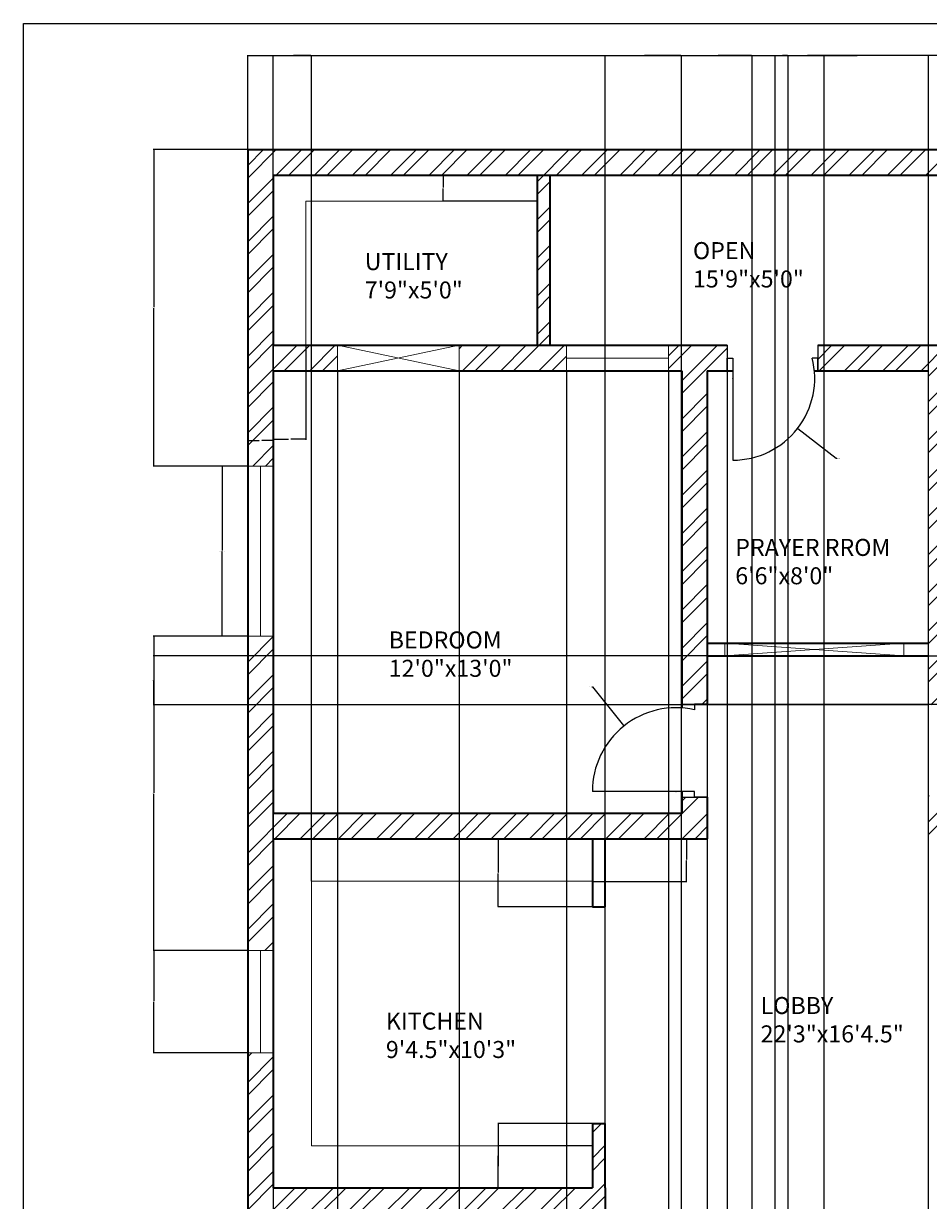
# Model space of a CAD drawing. Units: inches. Extents: x 1595 to 2135, y 460 to 2061.
# Tile 4 of 5: x 1595 to 1914, y 1646 to 2061. Entities that reach past the tile are written whole.
import ezdxf

# ---------------------------------------------------------------- set-up
doc = ezdxf.new("R2010")
doc.units = ezdxf.units.IN
for name, color, linetype, lineweight in [('A-ANNO-DIMS', 2, 'Continuous', 18), ('A-ANNO-TTLB', 7, 'Continuous', 25), ('A-AREA-IDEN', 7, 'Continuous', 18), ('A-DOOR', 3, 'Continuous', 25), ('A-FLOR-FIXT', 9, 'Continuous', 18), ('A-GLAZ', 4, 'Continuous', 18), ('A-WALL', 7, 'Continuous', 35)]:
    doc.layers.add(name, color=color, linetype=linetype, lineweight=lineweight)
doc.layers.add('A-WALL-PATT', color=143, linetype='Continuous', lineweight=13, true_color=0x7aafdf)
doc.styles.get("Standard").update_dxf_attribs({"font": 'arial.ttf'})
doc.dimstyles.get("Standard").update_dxf_attribs({"dimtxt": 0.18, "dimasz": 0.18, "dimexe": 0.18, "dimexo": 0.0625, "dimgap": 0.09, "dimtad": 0, "dimtih": 1, "dimtoh": 1, "dimdec": 4, "dimzin": 0, "dimdsep": 46, "dimtxsty": 'Standard', "dimcen": 0.09, "dimadec": 0, "dimazin": 0, "dimtfac": 1, "dimtdec": 4, "dimtofl": 0, "dimtmove": 0, "dimatfit": 3, "dimfxl": 1, "dimtolj": 1, "dimtzin": 0, "dimarcsym": 0})

# ---------------------------------------------------------------- blocks, each defined once
blk = doc.blocks.new('WIN-60IN')
for p, q in [((4.5, 60), (0, 60)), ((0, 60), (9, 60)), ((4.5, 0), (4.5, 60)), ((0, 0), (9, 0)), ((9, 0), (4.5, 0))]:
    blk.add_line(p, q)
blk = doc.blocks.new('*D2')
at = {"layer": 'A-ANNO-DIMS', "color": 0, "lineweight": -2, "transparency": 16777216}
for p, q in [((1674.25, 1905.07), (1665.13, 1905.07)), ((1665.31, 1904.89), (1665.31, 1875.26)), ((1665.31, 1845.25), (1665.31, 1874.89)), ((1674.25, 1845.07), (1665.13, 1845.07))]:
    blk.add_line(p, q, dxfattribs=at)
at = {"layer": 'A-ANNO-DIMS', "color": 0, "transparency": 16777216}
for points in [[(1665.28, 1904.89), (1665.34, 1904.89), (1665.31, 1905.07)], [(1665.28, 1845.25), (1665.34, 1845.25), (1665.31, 1845.07)]]:
    blk.add_solid(points, dxfattribs=at)
at = {"layer": 'Defpoints', "color": 0, "transparency": 16777216}
for p in [(1674.31, 1905.07), (1665.31, 1845.07), (1674.31, 1845.07)]:
    blk.add_point(p, dxfattribs=at)
at = {"layer": 'A-ANNO-DIMS', "color": 0, "transparency": 16777216, "insert": (1665.31, 1875.07), "char_height": 0.18, "attachment_point": 5}
blk.add_mtext('\\A1;WINDOW 60 TYP.', dxfattribs=at)
blk = doc.blocks.new('*D3')
at = {"layer": 'A-ANNO-DIMS', "color": 0, "lineweight": -2, "transparency": 16777216}
for p, q in [((1674.31, 1905.14), (1674.31, 1914.25)), ((1674.49, 1914.07), (1678.35, 1914.07)), ((1683.13, 1914.07), (1679.27, 1914.07)), ((1683.31, 1905.14), (1683.31, 1914.25))]:
    blk.add_line(p, q, dxfattribs=at)
at = {"layer": 'A-ANNO-DIMS', "color": 0, "transparency": 16777216}
for points in [[(1674.49, 1914.1), (1674.49, 1914.04), (1674.31, 1914.07)], [(1683.13, 1914.1), (1683.13, 1914.04), (1683.31, 1914.07)]]:
    blk.add_solid(points, dxfattribs=at)
at = {"layer": 'Defpoints', "color": 0, "transparency": 16777216}
for p in [(1674.31, 1914.07), (1674.31, 1905.07), (1683.31, 1905.07)]:
    blk.add_point(p, dxfattribs=at)
at = {"layer": 'A-ANNO-DIMS', "color": 0, "transparency": 16777216, "insert": (1678.81, 1914.07), "char_height": 0.18, "attachment_point": 5}
blk.add_mtext('\\A1;9 TYP.', dxfattribs=at)
blk = doc.blocks.new('*D4')
at = {"layer": 'A-ANNO-DIMS', "color": 0, "lineweight": -2, "transparency": 16777216}
for p, q in [((1795.75, 1773.64), (1762.48, 1773.64)), ((1762.66, 1773.46), (1762.66, 1761.82)), ((1762.66, 1749.81), (1762.66, 1761.46)), ((1795.75, 1749.63), (1762.48, 1749.63))]:
    blk.add_line(p, q, dxfattribs=at)
at = {"layer": 'A-ANNO-DIMS', "color": 0, "transparency": 16777216}
for points in [[(1762.63, 1773.46), (1762.69, 1773.46), (1762.66, 1773.64)], [(1762.63, 1749.81), (1762.69, 1749.81), (1762.66, 1749.63)]]:
    blk.add_solid(points, dxfattribs=at)
at = {"layer": 'Defpoints', "color": 0, "transparency": 16777216}
for p in [(1762.66, 1773.64), (1795.81, 1773.64), (1795.81, 1749.63)]:
    blk.add_point(p, dxfattribs=at)
at = {"layer": 'A-ANNO-DIMS', "color": 0, "transparency": 16777216, "insert": (1762.66, 1761.64), "char_height": 0.18, "attachment_point": 5}
blk.add_mtext('\\A1;24.01', dxfattribs=at)
blk = doc.blocks.new('*D5')
at = {"layer": 'A-ANNO-DIMS', "color": 0, "lineweight": -2, "transparency": 16777216}
for p, q in [((1795.75, 1673.31), (1762.48, 1673.31)), ((1762.66, 1673.13), (1762.66, 1662.16)), ((1762.66, 1650.82), (1762.66, 1661.79)), ((1795.75, 1650.64), (1762.48, 1650.64))]:
    blk.add_line(p, q, dxfattribs=at)
at = {"layer": 'A-ANNO-DIMS', "color": 0, "transparency": 16777216}
for points in [[(1762.63, 1673.13), (1762.69, 1673.13), (1762.66, 1673.31)], [(1762.63, 1650.82), (1762.69, 1650.82), (1762.66, 1650.64)]]:
    blk.add_solid(points, dxfattribs=at)
at = {"layer": 'Defpoints', "color": 0, "transparency": 16777216}
for p in [(1762.66, 1673.31), (1795.81, 1673.31), (1795.81, 1650.64)]:
    blk.add_point(p, dxfattribs=at)
at = {"layer": 'A-ANNO-DIMS', "color": 0, "transparency": 16777216, "insert": (1762.66, 1661.97), "char_height": 0.18, "attachment_point": 5}
blk.add_mtext('\\A1;22.663', dxfattribs=at)
blk = doc.blocks.new('*D11')
at = {"layer": 'A-ANNO-DIMS', "color": 0, "lineweight": -2, "transparency": 16777216}
for p, q in [((1674.25, 2016.64), (1640.98, 2016.64)), ((1641.16, 2016.46), (1641.16, 1961.04)), ((1641.16, 1905.25), (1641.16, 1960.68)), ((1674.25, 1905.07), (1640.98, 1905.07))]:
    blk.add_line(p, q, dxfattribs=at)
at = {"layer": 'A-ANNO-DIMS', "color": 0, "transparency": 16777216}
for points in [[(1641.13, 2016.46), (1641.19, 2016.46), (1641.16, 2016.64)], [(1641.13, 1905.25), (1641.19, 1905.25), (1641.16, 1905.07)]]:
    blk.add_solid(points, dxfattribs=at)
at = {"layer": 'Defpoints', "color": 0, "transparency": 16777216}
for p in [(1674.31, 2016.64), (1641.16, 1905.07), (1674.31, 1905.07)]:
    blk.add_point(p, dxfattribs=at)
at = {"layer": 'A-ANNO-DIMS', "color": 0, "transparency": 16777216, "insert": (1641.16, 1960.86), "char_height": 0.18, "attachment_point": 5}
blk.add_mtext('\\A1;111.57', dxfattribs=at)
blk = doc.blocks.new('*D12')
at = {"layer": 'A-ANNO-DIMS', "color": 0, "lineweight": -2, "transparency": 16777216}
for p, q in [((1674.25, 1734.21), (1640.98, 1734.21)), ((1641.16, 1734.03), (1641.16, 1716.39)), ((1641.16, 1698.39), (1641.16, 1716.03)), ((1674.25, 1698.21), (1640.98, 1698.21))]:
    blk.add_line(p, q, dxfattribs=at)
at = {"layer": 'A-ANNO-DIMS', "color": 0, "transparency": 16777216}
for points in [[(1641.13, 1734.03), (1641.19, 1734.03), (1641.16, 1734.21)], [(1641.13, 1698.39), (1641.19, 1698.39), (1641.16, 1698.21)]]:
    blk.add_solid(points, dxfattribs=at)
at = {"layer": 'Defpoints', "color": 0, "transparency": 16777216}
for p in [(1674.31, 1734.21), (1641.16, 1698.21), (1674.31, 1698.21)]:
    blk.add_point(p, dxfattribs=at)
at = {"layer": 'A-ANNO-DIMS', "color": 0, "transparency": 16777216, "insert": (1641.16, 1716.21), "char_height": 0.18, "attachment_point": 5}
blk.add_mtext('\\A1;36', dxfattribs=at)
blk = doc.blocks.new('*D13')
at = {"layer": 'A-ANNO-DIMS', "color": 0, "lineweight": -2, "transparency": 16777216}
for p, q in [((1674.25, 1845.07), (1640.98, 1845.07)), ((1641.16, 1844.89), (1641.16, 1789.82)), ((1641.16, 1734.39), (1641.16, 1789.46)), ((1674.25, 1734.21), (1640.98, 1734.21))]:
    blk.add_line(p, q, dxfattribs=at)
at = {"layer": 'A-ANNO-DIMS', "color": 0, "transparency": 16777216}
for points in [[(1641.13, 1844.89), (1641.19, 1844.89), (1641.16, 1845.07)], [(1641.13, 1734.39), (1641.19, 1734.39), (1641.16, 1734.21)]]:
    blk.add_solid(points, dxfattribs=at)
at = {"layer": 'Defpoints', "color": 0, "transparency": 16777216}
for p in [(1674.31, 1845.07), (1641.16, 1734.21), (1674.31, 1734.21)]:
    blk.add_point(p, dxfattribs=at)
at = {"layer": 'A-ANNO-DIMS', "color": 0, "transparency": 16777216, "insert": (1641.16, 1789.64), "char_height": 0.18, "attachment_point": 5}
blk.add_mtext('\\A1;110.86', dxfattribs=at)
blk = doc.blocks.new('*D23')
at = {"layer": 'A-ANNO-DIMS', "color": 0, "lineweight": -2, "transparency": 16777216}
for p, q in [((1683.31, 1938.58), (1683.31, 1365.31)), ((1705.98, 1938.58), (1705.98, 1365.31)), ((1683.49, 1365.49), (1694.18, 1365.49)), ((1705.8, 1365.49), (1695.11, 1365.49))]:
    blk.add_line(p, q, dxfattribs=at)
at = {"layer": 'A-ANNO-DIMS', "color": 0, "transparency": 16777216}
for points in [[(1683.49, 1365.52), (1683.49, 1365.46), (1683.31, 1365.49)], [(1705.8, 1365.52), (1705.8, 1365.46), (1705.98, 1365.49)]]:
    blk.add_solid(points, dxfattribs=at)
at = {"layer": 'Defpoints', "color": 0, "transparency": 16777216}
for p in [(1683.31, 1938.64), (1705.98, 1938.64), (1705.98, 1365.49)]:
    blk.add_point(p, dxfattribs=at)
at = {"layer": 'A-ANNO-DIMS', "color": 0, "transparency": 16777216, "insert": (1694.64, 1365.49), "char_height": 0.18, "attachment_point": 5}
blk.add_mtext('\\A1;22.663', dxfattribs=at)
blk = doc.blocks.new('*D24')
at = {"layer": 'A-ANNO-DIMS', "color": 0, "lineweight": -2, "transparency": 16777216}
for p, q in [((1705.98, 1938.58), (1705.98, 1365.31)), ((1748.87, 1938.58), (1748.87, 1365.31)), ((1706.16, 1365.49), (1726.96, 1365.49)), ((1748.69, 1365.49), (1727.89, 1365.49))]:
    blk.add_line(p, q, dxfattribs=at)
at = {"layer": 'A-ANNO-DIMS', "color": 0, "transparency": 16777216}
for points in [[(1706.16, 1365.52), (1706.16, 1365.46), (1705.98, 1365.49)], [(1748.69, 1365.52), (1748.69, 1365.46), (1748.87, 1365.49)]]:
    blk.add_solid(points, dxfattribs=at)
at = {"layer": 'Defpoints', "color": 0, "transparency": 16777216}
for p in [(1705.98, 1938.64), (1748.87, 1938.64), (1748.87, 1365.49)]:
    blk.add_point(p, dxfattribs=at)
at = {"layer": 'A-ANNO-DIMS', "color": 0, "transparency": 16777216, "insert": (1727.42, 1365.49), "char_height": 0.18, "attachment_point": 5}
blk.add_mtext('\\A1;42.894', dxfattribs=at)
blk = doc.blocks.new('*D25')
at = {"layer": 'A-ANNO-DIMS', "color": 0, "lineweight": -2, "transparency": 16777216}
for p, q in [((1748.87, 1938.58), (1748.87, 1365.31)), ((1786.65, 1938.58), (1786.65, 1365.31)), ((1749.05, 1365.49), (1767.37, 1365.49)), ((1786.47, 1365.49), (1768.16, 1365.49))]:
    blk.add_line(p, q, dxfattribs=at)
at = {"layer": 'A-ANNO-DIMS', "color": 0, "transparency": 16777216}
for points in [[(1749.05, 1365.52), (1749.05, 1365.46), (1748.87, 1365.49)], [(1786.47, 1365.52), (1786.47, 1365.46), (1786.65, 1365.49)]]:
    blk.add_solid(points, dxfattribs=at)
at = {"layer": 'Defpoints', "color": 0, "transparency": 16777216}
for p in [(1748.87, 1938.64), (1786.65, 1938.64), (1786.65, 1365.49)]:
    blk.add_point(p, dxfattribs=at)
at = {"layer": 'A-ANNO-DIMS', "color": 0, "transparency": 16777216, "insert": (1767.76, 1365.49), "char_height": 0.18, "attachment_point": 5}
blk.add_mtext('\\A1;37.78', dxfattribs=at)
blk = doc.blocks.new('*D26')
at = {"layer": 'A-ANNO-DIMS', "color": 0, "lineweight": -2, "transparency": 16777216}
for p, q in [((1786.65, 1938.58), (1786.65, 1365.31)), ((1822.65, 1938.58), (1822.65, 1365.31)), ((1786.83, 1365.49), (1804.43, 1365.49)), ((1822.47, 1365.49), (1804.87, 1365.49))]:
    blk.add_line(p, q, dxfattribs=at)
at = {"layer": 'A-ANNO-DIMS', "color": 0, "transparency": 16777216}
for points in [[(1786.83, 1365.52), (1786.83, 1365.46), (1786.65, 1365.49)], [(1822.47, 1365.52), (1822.47, 1365.46), (1822.65, 1365.49)]]:
    blk.add_solid(points, dxfattribs=at)
at = {"layer": 'Defpoints', "color": 0, "transparency": 16777216}
for p in [(1786.65, 1938.64), (1822.65, 1938.64), (1822.65, 1365.49)]:
    blk.add_point(p, dxfattribs=at)
at = {"layer": 'A-ANNO-DIMS', "color": 0, "transparency": 16777216, "insert": (1804.65, 1365.49), "char_height": 0.18, "attachment_point": 5}
blk.add_mtext('\\A1;36', dxfattribs=at)
blk = doc.blocks.new('*D30')
at = {"layer": 'A-ANNO-DIMS', "color": 0, "lineweight": -2, "transparency": 16777216}
for p, q in [((1836.31, 1938.58), (1836.31, 1365.31)), ((1843.37, 1938.58), (1843.37, 1365.31)), ((1836.49, 1365.49), (1839.45, 1365.49)), ((1843.19, 1365.49), (1840.23, 1365.49))]:
    blk.add_line(p, q, dxfattribs=at)
at = {"layer": 'A-ANNO-DIMS', "color": 0, "transparency": 16777216}
for points in [[(1836.49, 1365.52), (1836.49, 1365.46), (1836.31, 1365.49)], [(1843.19, 1365.52), (1843.19, 1365.46), (1843.37, 1365.49)]]:
    blk.add_solid(points, dxfattribs=at)
at = {"layer": 'Defpoints', "color": 0, "transparency": 16777216}
for p in [(1836.31, 1938.64), (1843.37, 1938.64), (1843.37, 1365.49)]:
    blk.add_point(p, dxfattribs=at)
at = {"layer": 'A-ANNO-DIMS', "color": 0, "transparency": 16777216, "insert": (1839.84, 1365.49), "char_height": 0.18, "attachment_point": 5}
blk.add_mtext('\\A1;7.054', dxfattribs=at)
blk = doc.blocks.new('*D31')
at = {"layer": 'A-ANNO-DIMS', "color": 0, "lineweight": -2, "transparency": 16777216}
for p, q in [((1836.38, 1838.14), (2109.64, 1838.14)), ((2109.46, 1837.96), (2109.46, 1829.81)), ((2109.46, 1821.29), (2109.46, 1829.44)), ((1836.38, 1821.11), (2109.64, 1821.11))]:
    blk.add_line(p, q, dxfattribs=at)
at = {"layer": 'A-ANNO-DIMS', "color": 0, "transparency": 16777216}
for points in [[(2109.43, 1837.96), (2109.49, 1837.96), (2109.46, 1838.14)], [(2109.43, 1821.29), (2109.49, 1821.29), (2109.46, 1821.11)]]:
    blk.add_solid(points, dxfattribs=at)
at = {"layer": 'Defpoints', "color": 0, "transparency": 16777216}
for p in [(1836.31, 1838.14), (1836.31, 1821.11), (2109.46, 1821.11)]:
    blk.add_point(p, dxfattribs=at)
at = {"layer": 'A-ANNO-DIMS', "color": 0, "transparency": 16777216, "insert": (2109.46, 1829.63), "char_height": 0.18, "attachment_point": 5}
blk.add_mtext('\\A1;17.034', dxfattribs=at)
blk = doc.blocks.new('*D32')
at = {"layer": 'A-ANNO-DIMS', "color": 0, "lineweight": -2, "transparency": 16777216}
for p, q in [((1914.25, 1838.14), (1640.98, 1838.14)), ((1641.16, 1837.96), (1641.16, 1829.7)), ((1641.16, 1821.07), (1641.16, 1829.33)), ((1914.25, 1820.89), (1640.98, 1820.89))]:
    blk.add_line(p, q, dxfattribs=at)
at = {"layer": 'A-ANNO-DIMS', "color": 0, "transparency": 16777216}
for points in [[(1641.13, 1837.96), (1641.19, 1837.96), (1641.16, 1838.14)], [(1641.13, 1821.07), (1641.19, 1821.07), (1641.16, 1820.89)]]:
    blk.add_solid(points, dxfattribs=at)
at = {"layer": 'Defpoints', "color": 0, "transparency": 16777216}
for p in [(1914.31, 1838.14), (1641.16, 1820.89), (1914.31, 1820.89)]:
    blk.add_point(p, dxfattribs=at)
at = {"layer": 'A-ANNO-DIMS', "color": 0, "transparency": 16777216, "insert": (1641.16, 1829.52), "char_height": 0.18, "attachment_point": 5}
blk.add_mtext('\\A1;17.253', dxfattribs=at)
blk = doc.blocks.new('*D35')
at = {"layer": 'A-ANNO-DIMS', "color": 0, "lineweight": -2, "transparency": 16777216}
for p, q in [((1864.81, 1540.04), (1864.81, 2049.97)), ((1864.99, 2049.79), (1889.23, 2049.79)), ((1914.13, 2049.79), (1889.89, 2049.79)), ((1914.31, 1540.04), (1914.31, 2049.97))]:
    blk.add_line(p, q, dxfattribs=at)
at = {"layer": 'A-ANNO-DIMS', "color": 0, "transparency": 16777216}
for points in [[(1864.99, 2049.82), (1864.99, 2049.76), (1864.81, 2049.79)], [(1914.13, 2049.82), (1914.13, 2049.76), (1914.31, 2049.79)]]:
    blk.add_solid(points, dxfattribs=at)
at = {"layer": 'Defpoints', "color": 0, "transparency": 16777216}
for p in [(1914.31, 2049.79), (1864.81, 1539.98), (1914.31, 1539.98)]:
    blk.add_point(p, dxfattribs=at)
at = {"layer": 'A-ANNO-DIMS', "color": 0, "transparency": 16777216, "insert": (1889.56, 2049.79), "char_height": 0.18, "attachment_point": 5}
blk.add_mtext('\\A1;49.5', dxfattribs=at)
blk = doc.blocks.new('*D36')
at = {"layer": 'A-ANNO-DIMS', "color": 0, "lineweight": -2, "transparency": 16777216}
for p, q in [((1860.31, 1568.2), (1860.31, 2049.97)), ((1860.49, 2049.79), (1862.3, 2049.79)), ((1864.63, 2049.79), (1862.82, 2049.79)), ((1864.81, 1577.2), (1864.81, 2049.97))]:
    blk.add_line(p, q, dxfattribs=at)
at = {"layer": 'A-ANNO-DIMS', "color": 0, "transparency": 16777216}
for points in [[(1860.49, 2049.82), (1860.49, 2049.76), (1860.31, 2049.79)], [(1864.63, 2049.82), (1864.63, 2049.76), (1864.81, 2049.79)]]:
    blk.add_solid(points, dxfattribs=at)
at = {"layer": 'Defpoints', "color": 0, "transparency": 16777216}
for p in [(1864.81, 2049.79), (1864.81, 1577.14), (1860.31, 1568.14)]:
    blk.add_point(p, dxfattribs=at)
at = {"layer": 'A-ANNO-DIMS', "color": 0, "transparency": 16777216, "insert": (1862.56, 2049.79), "char_height": 0.18, "attachment_point": 5}
blk.add_mtext('\\A1;4.5', dxfattribs=at)
blk = doc.blocks.new('*D37')
at = {"layer": 'A-ANNO-DIMS', "color": 0, "lineweight": -2, "transparency": 16777216}
for p, q in [((1800.31, 1577.2), (1800.31, 2049.97)), ((1800.49, 2049.79), (1813.31, 2049.79)), ((1827.06, 2049.79), (1814.24, 2049.79)), ((1827.24, 1577.2), (1827.24, 2049.97))]:
    blk.add_line(p, q, dxfattribs=at)
at = {"layer": 'A-ANNO-DIMS', "color": 0, "transparency": 16777216}
for points in [[(1800.49, 2049.82), (1800.49, 2049.76), (1800.31, 2049.79)], [(1827.06, 2049.82), (1827.06, 2049.76), (1827.24, 2049.79)]]:
    blk.add_solid(points, dxfattribs=at)
at = {"layer": 'Defpoints', "color": 0, "transparency": 16777216}
for p in [(1827.24, 2049.79), (1800.31, 1577.14), (1827.24, 1577.14)]:
    blk.add_point(p, dxfattribs=at)
at = {"layer": 'A-ANNO-DIMS', "color": 0, "transparency": 16777216, "insert": (1813.78, 2049.79), "char_height": 0.18, "attachment_point": 5}
blk.add_mtext('\\A1;26.927', dxfattribs=at)
blk = doc.blocks.new('*D38')
at = {"layer": 'A-ANNO-DIMS', "color": 0, "lineweight": -2, "transparency": 16777216}
for p, q in [((1827.24, 1577.2), (1827.24, 2049.97)), ((1827.42, 2049.79), (1839.23, 2049.79)), ((1851.96, 2049.79), (1840.16, 2049.79)), ((1852.14, 1577.2), (1852.14, 2049.97))]:
    blk.add_line(p, q, dxfattribs=at)
at = {"layer": 'A-ANNO-DIMS', "color": 0, "transparency": 16777216}
for points in [[(1827.42, 2049.82), (1827.42, 2049.76), (1827.24, 2049.79)], [(1851.96, 2049.82), (1851.96, 2049.76), (1852.14, 2049.79)]]:
    blk.add_solid(points, dxfattribs=at)
at = {"layer": 'Defpoints', "color": 0, "transparency": 16777216}
for p in [(1852.14, 2049.79), (1827.24, 1577.14), (1852.14, 1577.14)]:
    blk.add_point(p, dxfattribs=at)
at = {"layer": 'A-ANNO-DIMS', "color": 0, "transparency": 16777216, "insert": (1839.69, 2049.79), "char_height": 0.18, "attachment_point": 5}
blk.add_mtext('\\A1;24.904', dxfattribs=at)
blk = doc.blocks.new('*D44')
at = {"layer": 'A-ANNO-DIMS', "color": 0, "lineweight": -2, "transparency": 16777216}
for p, q in [((1864.81, 1549.04), (1864.81, 2049.97)), ((1864.99, 2049.79), (1870.74, 2049.79)), ((1877.4, 2049.79), (1871.65, 2049.79)), ((1877.58, 1549.04), (1877.58, 2049.97))]:
    blk.add_line(p, q, dxfattribs=at)
at = {"layer": 'A-ANNO-DIMS', "color": 0, "transparency": 16777216}
for points in [[(1864.99, 2049.82), (1864.99, 2049.76), (1864.81, 2049.79)], [(1877.4, 2049.82), (1877.4, 2049.76), (1877.58, 2049.79)]]:
    blk.add_solid(points, dxfattribs=at)
at = {"layer": 'Defpoints', "color": 0, "transparency": 16777216}
for p in [(1877.58, 2049.79), (1864.81, 1548.98), (1877.58, 1548.98)]:
    blk.add_point(p, dxfattribs=at)
at = {"layer": 'A-ANNO-DIMS', "color": 0, "transparency": 16777216, "insert": (1871.2, 2049.79), "char_height": 0.18, "attachment_point": 5}
blk.add_mtext('\\A1;12.769', dxfattribs=at)
blk = doc.blocks.new('*D45')
at = {"layer": 'A-ANNO-DIMS', "color": 0, "lineweight": -2, "transparency": 16777216}
for p, q in [((1674.31, 2016.7), (1674.31, 2049.97)), ((1674.49, 2049.79), (1875.02, 2049.79)), ((2076.13, 2049.79), (1875.6, 2049.79)), ((2076.31, 2016.7), (2076.31, 2049.97))]:
    blk.add_line(p, q, dxfattribs=at)
at = {"layer": 'A-ANNO-DIMS', "color": 0, "transparency": 16777216}
for points in [[(1674.49, 2049.82), (1674.49, 2049.76), (1674.31, 2049.79)], [(2076.13, 2049.82), (2076.13, 2049.76), (2076.31, 2049.79)]]:
    blk.add_solid(points, dxfattribs=at)
at = {"layer": 'Defpoints', "color": 0, "transparency": 16777216}
for p in [(2076.31, 2049.79), (1674.31, 2016.64), (2076.31, 2016.64)]:
    blk.add_point(p, dxfattribs=at)
at = {"layer": 'A-ANNO-DIMS', "color": 0, "transparency": 16777216, "insert": (1875.31, 2049.79), "char_height": 0.18, "attachment_point": 5}
blk.add_mtext('\\A1;402', dxfattribs=at)
blk = doc.blocks.new('*D49')
at = {"layer": 'A-ANNO-DIMS', "color": 0, "lineweight": -2, "transparency": 16777216}
for p, q in [((1683.31, 1947.58), (1683.31, 1914.31)), ((1694.85, 1947.58), (1694.85, 1914.31)), ((1683.49, 1914.49), (1688.7, 1914.49)), ((1694.67, 1914.49), (1689.47, 1914.49))]:
    blk.add_line(p, q, dxfattribs=at)
at = {"layer": 'A-ANNO-DIMS', "color": 0, "transparency": 16777216}
for points in [[(1683.49, 1914.52), (1683.49, 1914.46), (1683.31, 1914.49)], [(1694.67, 1914.52), (1694.67, 1914.46), (1694.85, 1914.49)]]:
    blk.add_solid(points, dxfattribs=at)
at = {"layer": 'Defpoints', "color": 0, "transparency": 16777216}
for p in [(1683.31, 1947.64), (1694.85, 1947.64), (1683.31, 1914.49)]:
    blk.add_point(p, dxfattribs=at)
at = {"layer": 'A-ANNO-DIMS', "color": 0, "transparency": 16777216, "insert": (1689.08, 1914.49), "char_height": 0.18, "attachment_point": 5}
blk.add_mtext('\\A1;11.54', dxfattribs=at)
blk = doc.blocks.new('*D50')
at = {"layer": 'A-ANNO-DIMS', "color": 0, "lineweight": -2, "transparency": 16777216}
for p, q in [((1776.25, 2007.64), (1742.98, 2007.64)), ((1743.16, 2007.46), (1743.16, 2003.24)), ((1743.16, 1998.65), (1743.16, 2002.87)), ((1776.25, 1998.47), (1742.98, 1998.47))]:
    blk.add_line(p, q, dxfattribs=at)
at = {"layer": 'A-ANNO-DIMS', "color": 0, "transparency": 16777216}
for points in [[(1743.13, 2007.46), (1743.19, 2007.46), (1743.16, 2007.64)], [(1743.13, 1998.65), (1743.19, 1998.65), (1743.16, 1998.47)]]:
    blk.add_solid(points, dxfattribs=at)
at = {"layer": 'Defpoints', "color": 0, "transparency": 16777216}
for p in [(1743.16, 2007.64), (1776.31, 2007.64), (1776.31, 1998.47)]:
    blk.add_point(p, dxfattribs=at)
at = {"layer": 'A-ANNO-DIMS', "color": 0, "transparency": 16777216, "insert": (1743.16, 2003.05), "char_height": 0.18, "attachment_point": 5}
blk.add_mtext('\\A1;9.175', dxfattribs=at)
blk = doc.blocks.new('*D53')
at = {"layer": 'A-ANNO-DIMS', "color": 0, "lineweight": -2, "transparency": 16777216}
for p, q in [((1683.31, 1773.7), (1683.31, 2049.97)), ((1683.49, 2049.79), (1689.66, 2049.79)), ((1696.59, 2049.79), (1690.43, 2049.79)), ((1696.77, 1758.72), (1696.77, 2049.97))]:
    blk.add_line(p, q, dxfattribs=at)
at = {"layer": 'A-ANNO-DIMS', "color": 0, "transparency": 16777216}
for points in [[(1683.49, 2049.82), (1683.49, 2049.76), (1683.31, 2049.79)], [(1696.59, 2049.82), (1696.59, 2049.76), (1696.77, 2049.79)]]:
    blk.add_solid(points, dxfattribs=at)
at = {"layer": 'Defpoints', "color": 0, "transparency": 16777216}
for p in [(1696.77, 2049.79), (1683.31, 1773.64), (1696.77, 1758.65)]:
    blk.add_point(p, dxfattribs=at)
at = {"layer": 'A-ANNO-DIMS', "color": 0, "transparency": 16777216, "insert": (1690.04, 2049.79), "char_height": 0.18, "attachment_point": 5}
blk.add_mtext('\\A1;13.46', dxfattribs=at)
blk = doc.blocks.new('*D54')
at = {"layer": 'A-ANNO-DIMS', "color": 0, "lineweight": -2, "transparency": 16777216}
for p, q in [((1795.88, 1773.64), (1829.14, 1773.64)), ((1828.96, 1773.46), (1828.96, 1766.33)), ((1828.96, 1758.83), (1828.96, 1765.97)), ((1795.88, 1758.65), (1829.14, 1758.65))]:
    blk.add_line(p, q, dxfattribs=at)
at = {"layer": 'A-ANNO-DIMS', "color": 0, "transparency": 16777216}
for points in [[(1828.93, 1773.46), (1828.99, 1773.46), (1828.96, 1773.64)], [(1828.93, 1758.83), (1828.99, 1758.83), (1828.96, 1758.65)]]:
    blk.add_solid(points, dxfattribs=at)
at = {"layer": 'Defpoints', "color": 0, "transparency": 16777216}
for p in [(1795.81, 1773.64), (1795.81, 1758.65), (1828.96, 1758.65)]:
    blk.add_point(p, dxfattribs=at)
at = {"layer": 'A-ANNO-DIMS', "color": 0, "transparency": 16777216, "insert": (1828.96, 1766.15), "char_height": 0.18, "attachment_point": 5}
blk.add_mtext('\\A1;14.99', dxfattribs=at)
blk = doc.blocks.new('*D55')
at = {"layer": 'A-ANNO-DIMS', "color": 0, "lineweight": -2, "transparency": 16777216}
for p, q in [((1795.75, 1665.35), (1762.48, 1665.35)), ((1762.66, 1665.17), (1762.66, 1658.18)), ((1762.66, 1650.82), (1762.66, 1657.82)), ((1795.75, 1650.64), (1762.48, 1650.64))]:
    blk.add_line(p, q, dxfattribs=at)
at = {"layer": 'A-ANNO-DIMS', "color": 0, "transparency": 16777216}
for points in [[(1762.63, 1665.17), (1762.69, 1665.17), (1762.66, 1665.35)], [(1762.63, 1650.82), (1762.69, 1650.82), (1762.66, 1650.64)]]:
    blk.add_solid(points, dxfattribs=at)
at = {"layer": 'Defpoints', "color": 0, "transparency": 16777216}
for p in [(1762.66, 1665.35), (1795.81, 1665.35), (1795.81, 1650.64)]:
    blk.add_point(p, dxfattribs=at)
at = {"layer": 'A-ANNO-DIMS', "color": 0, "transparency": 16777216, "insert": (1762.66, 1658), "char_height": 0.18, "attachment_point": 5}
blk.add_mtext('\\A1;14.71', dxfattribs=at)
blk = doc.blocks.new('*D56')
at = {"layer": 'A-ANNO-DIMS', "color": 0, "lineweight": -2, "transparency": 16777216}
for p, q in [((1795.68, 1827.22), (1795.86, 1827.22)), ((1795.86, 1827.22), (1806.78, 1813.54)), ((1825.2, 1790.36), (1825.38, 1790.36)), ((1825.29, 1790.27), (1825.29, 1790.45))]:
    blk.add_line(p, q, dxfattribs=at)
at = {"layer": 'A-ANNO-DIMS', "color": 0, "transparency": 16777216}
blk.add_solid([(1806.81, 1813.56), (1806.76, 1813.52), (1806.9, 1813.4)], dxfattribs=at)
at = {"layer": 'Defpoints', "color": 0, "transparency": 16777216}
for p in [(1806.9, 1813.4), (1825.29, 1790.36)]:
    blk.add_point(p, dxfattribs=at)
at = {"layer": 'A-ANNO-DIMS', "color": 0, "transparency": 16777216, "insert": (1795.13, 1827.22), "char_height": 0.18, "attachment_point": 5}
blk.add_mtext('\\A1;R29.476', dxfattribs=at)
blk = doc.blocks.new('*D58')
at = {"layer": 'A-ANNO-DIMS', "color": 0, "lineweight": -2, "transparency": 16777216}
for p, q in [((1845.28, 1935.99), (1845.46, 1935.99)), ((1845.37, 1935.9), (1845.37, 1936.08)), ((1881.83, 1907.69), (1868.3, 1918.19)), ((1882.01, 1907.69), (1881.83, 1907.69))]:
    blk.add_line(p, q, dxfattribs=at)
at = {"layer": 'A-ANNO-DIMS', "color": 0, "transparency": 16777216}
blk.add_solid([(1868.31, 1918.21), (1868.28, 1918.17), (1868.15, 1918.3)], dxfattribs=at)
at = {"layer": 'Defpoints', "color": 0, "transparency": 16777216}
for p in [(1845.37, 1935.99), (1868.15, 1918.3)]:
    blk.add_point(p, dxfattribs=at)
at = {"layer": 'A-ANNO-DIMS', "color": 0, "transparency": 16777216, "insert": (1882.56, 1907.69), "char_height": 0.18, "attachment_point": 5}
blk.add_mtext('\\A1;R28.847', dxfattribs=at)

msp = doc.modelspace()

# ---------------------------------------------------------------- hatches: boundary and pattern name
at = {"layer": 'A-WALL-PATT'}
h = msp.add_hatch(dxfattribs=at)
h.set_pattern_fill('ANSI32', color=256)
h.paths.add_polyline_path([(2076.313, 2016.6421), (1674.313, 2016.6421), (1674.313, 1905.0731), (1683.313, 1905.0731), (1683.313, 1938.6421), (1705.9756, 1938.6421), (1705.9756, 1947.6421), (1683.313, 1947.6421), (1683.313, 2007.6421), (2067.313, 2007.6421), (2067.313, 1947.6421), (2046.0304, 1947.6421), (2046.0304, 1938.6421), (2067.313, 1938.6421), (2067.313, 1906.0373), (2076.313, 1906.0373), (2076.313, 1947.6421)])
h.paths.add_polyline_path([(1786.653, 1947.6421), (1748.8699, 1947.6421), (1748.8699, 1938.6421), (1786.653, 1938.6421), (1786.653, 1943.1421)], flags=17)
h.paths.add_polyline_path([(1843.367, 1943.1421), (1843.367, 1947.6421), (1822.653, 1947.6421), (1822.653, 1938.6421), (1827.313, 1938.6421), (1827.313, 1821.1082), (1836.313, 1821.1082), (1836.313, 1938.6421), (1843.367, 1938.6421)])
h.paths.add_polyline_path([(1928.933, 1943.1421), (1928.933, 1947.6421), (1875.313, 1947.6421), (1875.313, 1938.6421), (1914.313, 1938.6421), (1914.313, 1820.8892), (1923.313, 1820.8892), (1923.313, 1938.6421), (1928.933, 1938.6421)])
h.paths.add_polyline_path([(1997.1133, 1947.6421), (1964.933, 1947.6421), (1964.933, 1938.6421), (1997.1133, 1938.6421)], flags=17)
h.paths.add_polyline_path([(1974.313, 2007.6421), (1969.813, 2007.6421), (1969.813, 1947.6421), (1974.313, 1947.6421)], flags=17)
h.paths.add_polyline_path([(1780.813, 2007.6421), (1776.313, 2007.6421), (1776.313, 1947.6421), (1780.813, 1947.6421)], flags=17)
h.paths.add_polyline_path([(1683.313, 1845.0731), (1674.313, 1845.0731), (1674.313, 1734.209), (1683.313, 1734.209), (1683.313, 1773.6421), (1795.813, 1773.6421), (1836.313, 1773.6421), (1836.313, 1788.3627), (1831.813, 1788.3627), (1827.313, 1788.3627), (1827.313, 1782.6421), (1683.313, 1782.6421)])
h.paths.add_polyline_path([(2076.313, 1846.0373), (2067.313, 1846.0373), (2067.313, 1782.6421), (1923.313, 1782.6421), (1923.313, 1788.8802), (1918.813, 1788.8802), (1914.313, 1788.8802), (1914.313, 1773.6421), (2067.313, 1773.6421), (2067.313, 1710.6421), (2076.313, 1710.6421)])
h.paths.add_polyline_path([(1844.0531, 1859.9747), (1909.4596, 1859.9747), (1909.4596, 1882.3635), (1844.0531, 1882.3635)], flags=9)
h.paths.add_polyline_path([(1721.6058, 1827.3507), (1768.2143, 1827.3507), (1768.2143, 1849.7395), (1721.6058, 1849.7395)], flags=9)
h.paths.add_polyline_path([(1786.8661, 1359.2872), (1978.2276, 1359.2872), (1978.2276, 1384.0157), (1786.8661, 1384.0157)], flags=9)
h.paths.add_polyline_path([(1795.7228, 1412.0413), (1871.5904, 1412.0413), (1871.5904, 1424.4055), (1795.7228, 1424.4055)], flags=9)
h.paths.add_polyline_path([(1954.3634, 1526.3976), (2013.549, 1526.3976), (2013.549, 1548.7864), (1954.3634, 1548.7864)], flags=9)
h.paths.add_polyline_path([(1871.0596, 1490.4707), (1913.1292, 1490.4707), (1913.1292, 1512.8595), (1871.0596, 1512.8595)], flags=9)
h.paths.add_polyline_path([(1810.9452, 1510.8402), (1845.9343, 1510.8402), (1845.9343, 1533.229), (1810.9452, 1533.229)], flags=9)
h.paths.add_polyline_path([(1720.9117, 1692.9695), (1767.819, 1692.9695), (1767.819, 1715.3583), (1720.9117, 1715.3583)], flags=9)
h.paths.add_polyline_path([(1853.0254, 1698.4614), (1904.6966, 1698.4614), (1904.6966, 1720.8503), (1853.0254, 1720.8503)], flags=9)
h.paths.add_polyline_path([(1970.399, 1827.3507), (2017.0075, 1827.3507), (2017.0075, 1849.7395), (1970.399, 1849.7395)], flags=9)
h.paths.add_polyline_path([(1994.3418, 1955.5613), (2029.5928, 1955.5613), (2029.5928, 1977.9501), (1994.3418, 1977.9501)], flags=25)
h.paths.add_polyline_path([(1828.8665, 1964.6116), (1868.5173, 1964.6116), (1868.5173, 1987.0004), (1828.8665, 1987.0004)], flags=25)
h.paths.add_polyline_path([(1698.1483, 1960.8371), (1733.3994, 1960.8371), (1733.3994, 1983.2259), (1698.1483, 1983.2259)], flags=25)
h = msp.add_hatch(dxfattribs=at)
h.set_pattern_fill('ANSI32', color=256)
h.paths.add_polyline_path([(1683.313, 1641.6421), (1791.313, 1641.6421), (1791.313, 1634.7169), (1800.313, 1634.7169), (1800.313, 1650.6421), (1800.313, 1673.3054), (1795.813, 1673.3054), (1795.813, 1650.6421), (1683.313, 1650.6421), (1683.313, 1698.209), (1678.813, 1698.209), (1674.313, 1698.209), (1674.313, 1398.6421), (1688.853, 1398.6421), (1688.853, 1403.1421), (1688.853, 1407.6421), (1683.313, 1407.6421)])
h.paths.add_polyline_path([(1800.313, 1568.1421), (1827.2399, 1568.1421), (1827.2399, 1572.6421), (1827.2399, 1577.1421), (1800.313, 1577.1421), (1800.313, 1604.9472), (1795.813, 1604.9472), (1791.313, 1604.9472), (1791.313, 1437.6421), (1800.313, 1437.6421), (1815.6708, 1437.6421), (1815.6708, 1442.1421), (1815.6708, 1446.6421), (1800.313, 1446.6421)])
h.paths.add_polyline_path([(1877.5816, 1545.4284), (1877.5816, 1548.9761), (1864.813, 1548.9761), (1864.813, 1577.1421), (1852.144, 1577.1421), (1852.144, 1568.1421), (1860.313, 1568.1421), (1860.313, 1446.6421), (1839.6708, 1446.6421), (1839.6708, 1437.6421), (1869.0647, 1437.6421), (1869.0647, 1442.1421), (1869.0647, 1446.6421), (1864.813, 1446.6421), (1864.813, 1539.9761), (1877.5816, 1539.9761), (1877.5816, 1541.8808)])
h.paths.add_polyline_path([(1923.313, 1568.1421), (1936.607, 1568.1421), (1936.607, 1577.1421), (1914.313, 1577.1421), (1914.313, 1548.9761), (1901.5816, 1548.9761), (1901.5816, 1539.9761), (1914.313, 1539.9761), (1914.313, 1446.6421), (1891.5684, 1446.6421), (1891.5684, 1437.6421), (1914.313, 1437.6421), (1923.313, 1437.6421)])
h.paths.add_polyline_path([(2067.313, 1577.1421), (2003.1294, 1577.1421), (2003.1294, 1568.1421), (2067.313, 1568.1421)])
h.paths.add_polyline_path([(2076.313, 1650.6421), (2067.313, 1650.6421), (2067.313, 1504.2035), (2076.313, 1504.2035)])
h.paths.add_polyline_path([(2076.313, 1444.2035), (2071.813, 1444.2035), (2067.313, 1444.2035), (2067.313, 1407.6421), (1923.313, 1407.6421), (1918.813, 1407.6421), (1914.313, 1407.6421), (1737.2767, 1407.6421), (1737.2767, 1398.6421), (2076.313, 1398.6421)])

# ---------------------------------------------------------------- linework, layer by layer
at = {"layer": 'A-ANNO-TTLB'}
msp.add_lwpolyline([(1595.2754, 2061.0707), (2134.6206, 2061.0707), (2134.6206, 1319.9937), (1595.2754, 1319.9937)], close=True, dxfattribs=at)
at = {"layer": 'A-DOOR'}
for p, q in [((1843.367, 1947.6421), (1843.367, 1938.6421)), ((1875.313, 1947.6421), (1875.313, 1938.6421)), ((1843.367, 1938.6421), (1843.367, 1943.1421)), ((1843.367, 1943.1421), (1845.367, 1943.1421)), ((1845.367, 1943.1421), (1845.367, 1907.1421)), ((1875.313, 1943.1421), (1873.313, 1943.1421)), ((1875.313, 1938.6421), (1875.313, 1943.1421)), ((1827.313, 1821.1082), (1836.313, 1821.1082)), ((1836.313, 1821.1082), (1831.813, 1821.1082)), ((1831.813, 1821.1082), (1831.813, 1819.1082)), ((1831.813, 1790.3627), (1795.813, 1790.3627)), ((1827.313, 1788.3627), (1827.313, 1788.3627)), ((1827.313, 1788.3627), (1836.313, 1788.3627)), ((1831.813, 1788.3627), (1831.813, 1790.3627)), ((1836.313, 1788.3627), (1831.813, 1788.3627))]:
    msp.add_line(p, q, dxfattribs=at)
for centre, radius, start, end in [((1845.367, 1935.989), 28.847, 270, 14.357079), ((1825.2895, 1790.3627), 29.4765, 77.213808, 180)]:
    msp.add_arc(centre, radius, start, end, dxfattribs=at)
at = {"layer": 'A-FLOR-FIXT'}
for p, q in [((1694.8523, 1947.6421), (1694.8523, 1998.4667)), ((1694.8523, 1998.4667), (1694.8523, 1998.4667)), ((1694.8523, 1998.4667), (1776.313, 1998.4667)), ((1795.813, 1758.6532), (1696.7727, 1758.6532)), ((1696.7727, 1758.6532), (1696.7727, 1665.3507)), ((1696.7727, 1665.3507), (1795.813, 1665.3507)), ((1795.813, 1665.3507), (1795.813, 1665.3507))]:
    msp.add_line(p, q, dxfattribs=at)
at = {"layer": 'A-GLAZ'}
for p, q in [((1705.9756, 1947.6421), (1705.9756, 1938.6421)), ((1748.8699, 1938.6421), (1705.9756, 1947.6421)), ((1705.9756, 1938.6421), (1748.8699, 1947.6421)), ((1748.8699, 1947.6421), (1748.8699, 1938.6421)), ((1786.653, 1947.6421), (1786.653, 1947.6421)), ((1786.653, 1947.6421), (1786.653, 1938.6421)), ((1822.653, 1943.1421), (1822.653, 1947.6421)), ((1822.653, 1947.6421), (1822.653, 1938.6421)), ((1786.653, 1938.6421), (1786.653, 1943.1421)), ((1786.653, 1943.1421), (1786.653, 1943.1421)), ((1786.653, 1943.1421), (1810.653, 1943.1421)), ((1810.653, 1943.1421), (1822.653, 1943.1421)), ((1822.653, 1938.6421), (1822.653, 1938.6421)), ((1842.4828, 1842.6421), (1842.4828, 1842.6421)), ((1842.4828, 1842.6421), (1842.4828, 1838.1421)), ((1842.4828, 1838.1421), (1905.6765, 1842.6421)), ((1905.6765, 1838.1421), (1842.4828, 1842.6421)), ((1905.6765, 1842.6421), (1905.6765, 1838.1421)), ((1683.313, 1734.209), (1674.313, 1734.209)), ((1678.813, 1698.209), (1678.813, 1734.209)), ((1678.813, 1734.209), (1683.313, 1734.209)), ((1674.313, 1698.209), (1683.313, 1698.209)), ((1683.313, 1698.209), (1678.813, 1698.209))]:
    msp.add_line(p, q, dxfattribs=at)
at = {"layer": 'A-WALL'}
for p, q in [((1674.313, 2016.6421), (2076.313, 2016.6421)), ((1674.313, 2016.6421), (1674.313, 1398.6421)), ((1683.313, 2007.6421), (2067.313, 2007.6421)), ((1683.313, 2007.6421), (1683.313, 1947.6421)), ((1776.313, 2007.6421), (1776.313, 1947.6421)), ((1780.813, 2007.6421), (1780.813, 1947.6421)), ((1683.313, 1947.6421), (1843.367, 1947.6421)), ((1875.313, 1947.6421), (2067.313, 1947.6421)), ((1683.313, 1938.6421), (1827.313, 1938.6421)), ((1683.313, 1938.6421), (1683.313, 1782.6421)), ((1827.313, 1938.6421), (1827.313, 1819.7696)), ((1836.313, 1938.6421), (1836.313, 1821.1082)), ((1836.313, 1938.6421), (1845.367, 1938.6421)), ((1874.0917, 1938.6421), (1914.313, 1938.6421)), ((1836.313, 1842.6421), (1914.313, 1842.6421)), ((1836.313, 1838.1421), (1914.313, 1838.1421)), ((1827.313, 1790.3627), (1827.313, 1782.6421)), ((1836.313, 1788.3627), (1836.313, 1773.6421)), ((1683.313, 1782.6421), (1827.313, 1782.6421)), ((1683.313, 1773.6421), (1836.313, 1773.6421)), ((1683.313, 1773.6421), (1683.313, 1650.6421)), ((1683.313, 1773.6421), (1795.813, 1773.6421)), ((1795.813, 1773.6421), (1795.813, 1749.6333)), ((1800.313, 1749.6333), (1800.313, 1773.6421)), ((1795.813, 1749.6333), (1800.313, 1749.6333)), ((1795.813, 1673.3054), (1800.313, 1673.3054)), ((1795.813, 1673.3054), (1795.813, 1650.6421)), ((1800.313, 1650.6421), (1800.313, 1673.3054)), ((1683.313, 1650.6421), (1795.813, 1650.6421)), ((1800.313, 1650.6421), (1800.313, 1634.7169))]:
    msp.add_line(p, q, dxfattribs=at)

# ---------------------------------------------------------------- block references
at = {"layer": 'A-GLAZ', "rotation": 180}
msp.add_blockref('WIN-60IN', (1683.3131, 1905.0736), dxfattribs=at)

# ---------------------------------------------------------------- texts
at = {"layer": 'A-AREA-IDEN', "char_height": 6, "attachment_point": 1}
for s, width, insert in [('OPEN\\P15\'9"x5\'0"', 138.533826, (1831.2792, 1984.0188)), ('UTILITY\\P7\'9"x5\'0"', 127.793896, (1715.5641, 1980.1379)), ('PRAYER RROM\\P6\'6"x8\'0"', 128.530953, (1846.1997, 1879.3819)), ('BEDROOM\\P12\'0"x13\'0"', 157.676153, (1724.0185, 1846.7579)), ('LOBBY\\P22\'3"x16\'4.5"', 147.969804, (1855.1393, 1717.8687)), ('KITCHEN\\P9\'4.5"x10\'3"', 197.865687, (1723.0256, 1712.3727))]:
    msp.add_mtext_dynamic_manual_height_columns(s, width=width, gutter_width=12.5, heights=[0], dxfattribs=dict(at, insert=insert))

# ---------------------------------------------------------------- dimensions: what is measured, and where the dimension line sits
at = {"layer": 'A-ANNO-DIMS'}
for base, p1, p2, override, picture, middle in [((2076.313, 2049.7921), (1674.313, 2016.6421), (2076.313, 2016.6421), {"dimdec": 0, "dimlfac": 1, "dimrnd": 0, "dimzin": 0, "dimdsep": 46, "dimlunit": 2}, '*D45', (1875.313, 2049.7921)), ((1696.7727, 2049.7921), (1683.313, 1773.6421), (1696.7727, 1758.6532), {"dimdec": 2, "dimlfac": 1, "dimrnd": 0, "dimzin": 0, "dimdsep": 46, "dimlunit": 2}, '*D53', (1690.0429, 2049.7921)), ((1827.2399, 2049.7921), (1800.313, 1577.1421), (1827.2399, 1577.1421), {"dimdec": 3, "dimlfac": 1, "dimrnd": 0, "dimzin": 0, "dimdsep": 46, "dimlunit": 2}, '*D37', (1813.7764, 2049.7921)), ((1852.144, 2049.7921), (1827.2399, 1577.1421), (1852.144, 1577.1421), {"dimdec": 3, "dimlfac": 1, "dimrnd": 0, "dimzin": 0, "dimdsep": 46, "dimlunit": 2}, '*D38', (1839.6919, 2049.7921)), ((1864.813, 2049.7921), (1860.313, 1568.1421), (1864.813, 1577.1421), {"dimdec": 1, "dimlfac": 1, "dimrnd": 0, "dimzin": 0, "dimdsep": 46, "dimlunit": 2}, '*D36', (1862.563, 2049.7921)), ((1914.313, 2049.7921), (1864.813, 1539.9761), (1914.313, 1539.9761), {"dimdec": 1, "dimlfac": 1, "dimrnd": 0, "dimzin": 0, "dimdsep": 46, "dimlunit": 2}, '*D35', (1889.563, 2049.7921)), ((1877.5816, 2049.7921), (1864.813, 1548.9761), (1877.5816, 1548.9761), {"dimdec": 3, "dimlfac": 1, "dimrnd": 0, "dimzin": 0, "dimdsep": 46, "dimlunit": 2}, '*D44', (1871.1973, 2049.7921)), ((1705.9756, 1365.4921), (1683.313, 1938.6421), (1705.9756, 1938.6421), {"dimdec": 3, "dimlfac": 1, "dimrnd": 0, "dimzin": 0, "dimdsep": 46, "dimlunit": 2}, '*D23', (1694.6443, 1365.4921)), ((1748.8699, 1365.4921), (1705.9756, 1938.6421), (1748.8699, 1938.6421), {"dimdec": 3, "dimlfac": 1, "dimrnd": 0, "dimzin": 0, "dimdsep": 46, "dimlunit": 2}, '*D24', (1727.4227, 1365.4921)), ((1786.653, 1365.4921), (1748.8699, 1938.6421), (1786.653, 1938.6421), {"dimdec": 2, "dimlfac": 1, "dimrnd": 0, "dimzin": 0, "dimdsep": 46, "dimlunit": 2}, '*D25', (1767.7614, 1365.4921)), ((1822.653, 1365.4921), (1786.653, 1938.6421), (1822.653, 1938.6421), {"dimdec": 0, "dimlfac": 1, "dimrnd": 0, "dimzin": 0, "dimdsep": 46, "dimlunit": 2}, '*D26', (1804.653, 1365.4921)), ((1843.367, 1365.4921), (1836.313, 1938.6421), (1843.367, 1938.6421), {"dimdec": 3, "dimlfac": 1, "dimrnd": 0, "dimzin": 0, "dimdsep": 46, "dimlunit": 2}, '*D30', (1839.84, 1365.4921))]:
    dim = msp.add_linear_dim(base=base, p1=p1, p2=p2, dimstyle='Standard', override=override, dxfattribs=at)
    dim.commit()
    dim.dimension.update_dxf_attribs({"geometry": picture, "text_midpoint": middle})
for base, p1, p2, angle, override, picture, middle in [((1641.163, 1905.0731), (1674.313, 2016.6421), (1674.313, 1905.0731), 90, {"dimdec": 2, "dimlfac": 1, "dimrnd": 0, "dimzin": 0, "dimdsep": 46, "dimlunit": 2}, '*D11', (1641.163, 1960.8576)), ((1743.163, 2007.6421), (1776.313, 1998.4667), (1776.313, 2007.6421), 90, {"dimdec": 3, "dimlfac": 1, "dimrnd": 0, "dimzin": 0, "dimdsep": 46, "dimlunit": 2}, '*D50', (1743.163, 2003.0544)), ((1683.313, 1914.4921), (1694.8523, 1947.6421), (1683.313, 1947.6421), 180, {"dimdec": 2, "dimlfac": 1, "dimrnd": 0, "dimzin": 0, "dimdsep": 46, "dimlunit": 2}, '*D49', (1689.0826, 1914.4921)), ((1641.163, 1734.209), (1674.313, 1845.0731), (1674.313, 1734.209), 90, {"dimdec": 2, "dimlfac": 1, "dimrnd": 0, "dimzin": 0, "dimdsep": 46, "dimlunit": 2}, '*D13', (1641.163, 1789.641)), ((1641.163, 1820.8892), (1914.313, 1838.1421), (1914.313, 1820.8892), 90, {"dimdec": 3, "dimlfac": 1, "dimrnd": 0, "dimzin": 0, "dimdsep": 46, "dimlunit": 2}, '*D32', (1641.163, 1829.5156)), ((2109.463, 1821.1082), (1836.313, 1838.1421), (1836.313, 1821.1082), 90, {"dimdec": 3, "dimlfac": 1, "dimrnd": 0, "dimzin": 0, "dimdsep": 46, "dimlunit": 2}, '*D31', (2109.463, 1829.6251)), ((1762.663, 1773.6421), (1795.813, 1749.6333), (1795.813, 1773.6421), 90, {"dimdec": 2, "dimlfac": 1, "dimrnd": 0, "dimzin": 0, "dimdsep": 46, "dimlunit": 2}, '*D4', (1762.663, 1761.6377)), ((1828.963, 1758.6532), (1795.813, 1773.6421), (1795.813, 1758.6532), 270, {"dimdec": 2, "dimlfac": 1, "dimrnd": 0, "dimzin": 0, "dimdsep": 46, "dimlunit": 2}, '*D54', (1828.963, 1766.1476)), ((1641.163, 1698.209), (1674.313, 1734.209), (1674.313, 1698.209), 90, {"dimdec": 0, "dimlfac": 1, "dimrnd": 0, "dimzin": 0, "dimdsep": 46, "dimlunit": 2}, '*D12', (1641.163, 1716.209)), ((1762.663, 1673.3054), (1795.813, 1650.6421), (1795.813, 1673.3054), 90, {"dimdec": 3, "dimlfac": 1, "dimrnd": 0, "dimzin": 0, "dimdsep": 46, "dimlunit": 2}, '*D5', (1762.663, 1661.9737)), ((1762.663, 1665.3507), (1795.813, 1650.6421), (1795.813, 1665.3507), 90, {"dimdec": 2, "dimlfac": 1, "dimrnd": 0, "dimzin": 0, "dimdsep": 46, "dimlunit": 2}, '*D55', (1762.663, 1657.9964))]:
    dim = msp.add_linear_dim(base=base, p1=p1, p2=p2, angle=angle, dimstyle='Standard', override=override, dxfattribs=at)
    dim.commit()
    dim.dimension.update_dxf_attribs({"geometry": picture, "text_midpoint": middle})
for center, mpoint, picture, middle in [((1845.367, 1935.989), (1868.154, 1918.3), '*D58', (1882.5559, 1907.6866)), ((1825.2895, 1790.3627), (1806.897, 1813.397), '*D56', (1795.1318, 1827.2176))]:
    dim = msp.add_radius_dim(center=center, mpoint=mpoint, dimstyle='Standard', override={"dimdec": 3, "dimlfac": 1, "dimrnd": 0, "dimzin": 0, "dimdsep": 46, "dimlunit": 2}, dxfattribs=at)
    dim.commit()
    dim.dimension.update_dxf_attribs({"geometry": picture, "text_midpoint": middle, "dimtype": 164})
for base, p1, p2, angle, text, picture, middle in [((1674.313, 1914.0731), (1683.313, 1905.0731), (1674.313, 1905.0731), 180, '<> TYP.', '*D3', (1678.813, 1914.0731)), ((1665.313, 1845.0731), (1674.313, 1905.0731), (1674.313, 1845.0731), 270, 'WINDOW <> TYP.', '*D2', (1665.313, 1875.0731))]:
    dim = msp.add_linear_dim(base=base, p1=p1, p2=p2, angle=angle, text=text, dimstyle='Standard', override={"dimdec": 0, "dimlfac": 1, "dimrnd": 0, "dimzin": 0, "dimdsep": 46, "dimlunit": 2}, dxfattribs=at)
    dim.commit()
    dim.dimension.update_dxf_attribs({"geometry": picture, "text_midpoint": middle})

doc.saveas('drawing.dxf')
